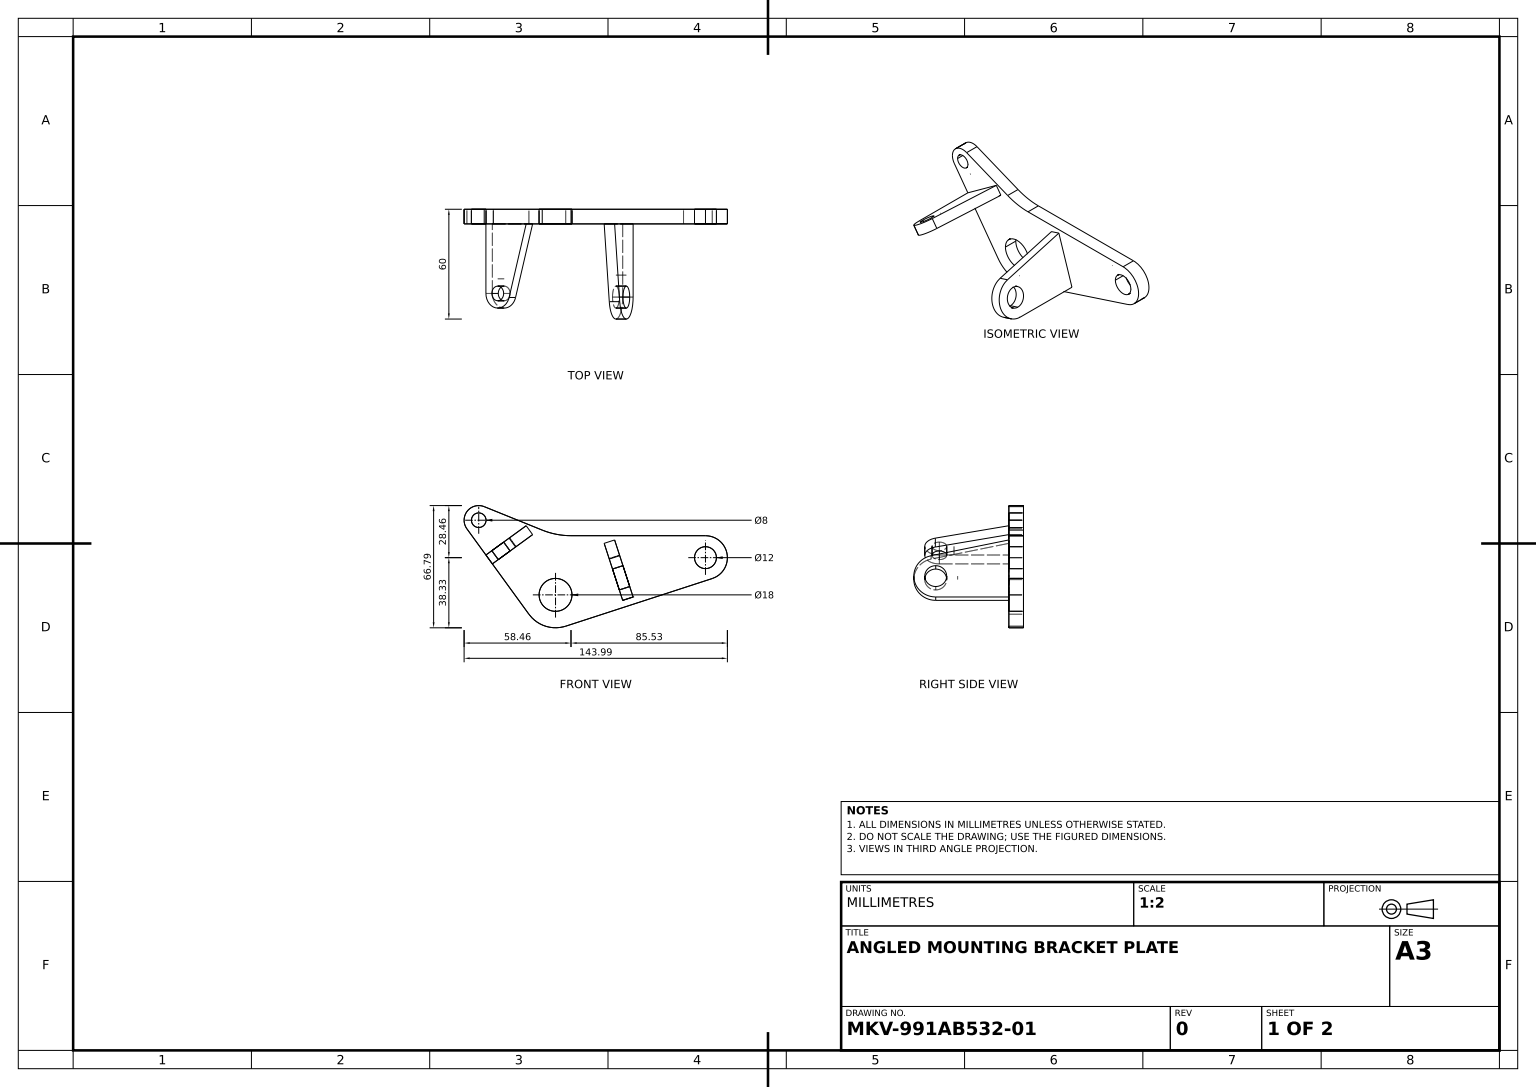
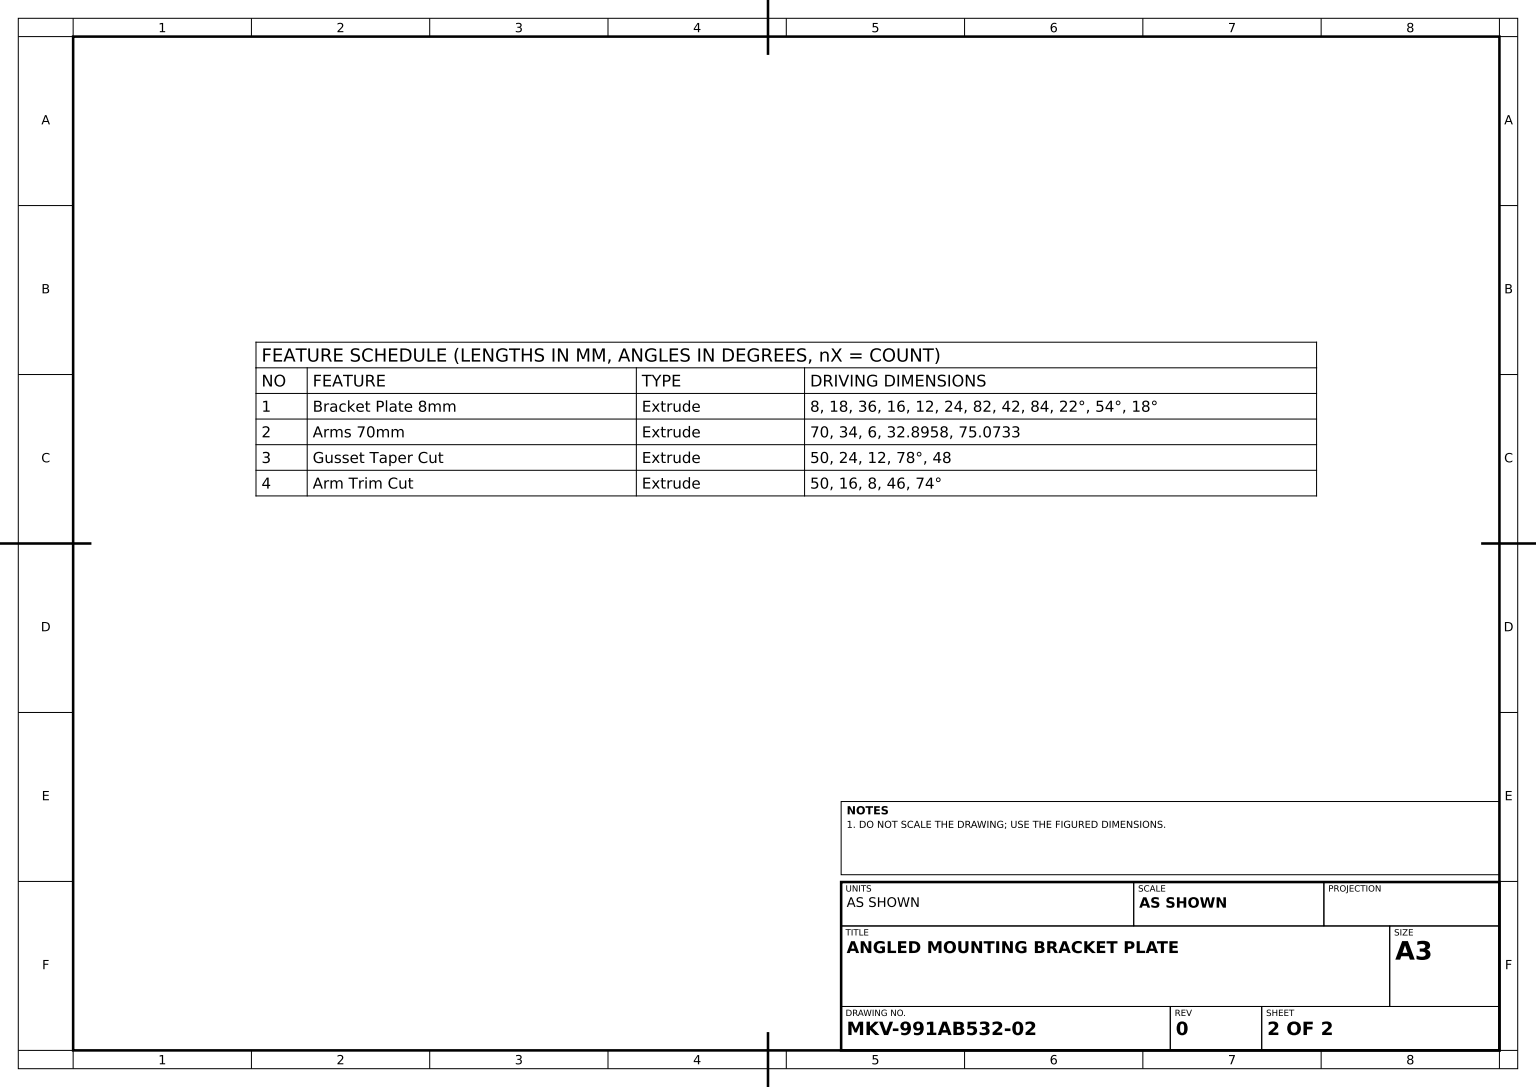
SolidWorks part; units mm, degrees
material "Plain Carbon Steel"
ref_plane "Front Plane" through (0, 0, 0) normal (0, 0, 1) x (1, 0, 0)
ref_plane "Top Plane" through (0, 0, 0) normal (0, 1, 0) x (1, 0, 0)
ref_plane "Right Plane" through (0, 0, 0) normal (1, 0, 0) x (0, 0, -1)
sketch "Bracket Plate Profile" plane through (0, 0, 0) normal (0, 0, 1) x (1, 0, 0)
  line L0 (-48.4721, 36.0927) -> (-14.5623, -10.5801)
  line L1 (5.5623, -17.119) -> (85.7082, 8.922)
  line L3 (-39.0031, 48.2125) -> (-7.2736, 35.3929)
  line L4 (8.4599, 32.3346) -> (82, 32.3346)
  circle A0 centre (0, 0) radius 9
  arc A1 (-14.5623, -10.5801) -> (5.5623, -17.119) centre (0, 0) ccw
  arc A2 (-39.0031, 48.2125) -> (-48.4721, 36.0927) centre (-42, 40.795) ccw
  circle A3 centre (-42, 40.795) radius 4
  arc A4 (85.7082, 8.922) -> (82, 32.3346) centre (82, 20.3346) ccw
  circle A5 centre (82, 20.3346) radius 6
  arc A6 (-7.2736, 35.3929) -> (8.4599, 32.3346) centre (8.4599, 74.3346) ccw
  dimension "D1" = 18
  dimension "D2" = 36
  dimension "D3" = 8
  dimension "D4" = 16
  dimension "D5" = 12
  dimension "D6" = 24
  dimension "D9" = 84
  dimension "D7" = 82
  dimension "D8" = 42
  dimension "D10" = 42
  dimension "D11" = 22
  dimension "D12" = 54
  dimension "D13" = 18
extrude "Bracket Plate 8mm" add sketch "Bracket Plate Profile" along normal blind 8
sketch "Arm Sections 34x6" plane through (0, 0, 8) normal (0, 0, 1) x (1, 0, 0)
  line L0 (37.8982, -6.6124) -> (43.6046, -4.7583)
  line L1 (37.8982, -6.6124) -> (26.6012, 28.1564)
  line L2 (43.6046, -4.7583) -> (32.3075, 30.0105)
  line L3 (26.6012, 28.1564) -> (32.3075, 30.0105)
  line L4 (-38.0737, 21.7805) -> (-34.547, 16.9264)
  line L5 (-38.0737, 21.7805) -> (-15.5763, 38.1259)
  line L6 (-34.547, 16.9264) -> (-12.0496, 33.2718)
  line L7 (-15.5763, 38.1259) -> (-12.0496, 33.2718)
  line L10 (-48.4721, 36.0927) -> (-14.5623, -10.5801) construction
  line L11 (5.5623, -17.119) -> (85.7082, 8.922) construction
  dimension "D1" = 34
  dimension "D2" = 6
  dimension "D3" = 34
  dimension "D4" = 6
  dimension "D5" = 32.8958
  dimension "D6" = 75.0733
extrude "Arms 70mm" add sketch "Arm Sections 34x6" along normal blind 70
sketch "Gusset Taper Cut Profile" plane through (38.0423, 12.3607, 0) normal (0.9511, 0.309, 0) x (0, 0, -1)
  line L0 (-8, 18.5581) -> (-50.4949, 9.5255)
  line L1 (-8, -14.2123) -> (-48, -14.2123)
  line L3 (-8, -18) -> (-8, 18.5581) construction
  line L8 (0, -18) -> (0, 5.4127) construction
  line L10 (-8, -18) -> (-8, 18.5581)
  line L11 (-8, 18.5581) -> (-78, 18.5581)
  line L12 (-78, 18.5581) -> (-78, -18)
  line L13 (-78, -18) -> (-8, -18)
  line L14 (-8, -18) -> (-8, 18.5581)
  line L15 (-8, 18.5581) -> (-78, 18.5581)
  line L16 (-78, 18.5581) -> (-78, -18)
  line L17 (-78, -18) -> (-8, -18)
  circle A0 centre (-48, -2.2123) radius 6
  arc A1 (-50.4949, 9.5255) -> (-48, -14.2123) centre (-48, -2.2123) ccw
  line M4 (-8, -18) -> (-8, 18.5581)
  line M5 (-8, 18.5581) -> (-78, 18.5581)
  line M6 (-78, 18.5581) -> (-78, -18)
  line M7 (-78, -18) -> (-8, -18)
  dimension "D1" = 24
  dimension "D2" = 12
  dimension "D3" = 78
  dimension "D4" = 48
  dimension "D5" = 0
extrude "Gusset Taper Cut" cut sketch "Gusset Taper Cut Profile" against normal blind 50 contours A1 L0 L1 M5 M6 M7 M4 | A0
sketch "Arm Trim Cut Profile" plane through (-23.5114, 32.3607, 0) normal (-0.5878, 0.809, 0) x (0.809, 0.5878, 0)
  line L0 (9.2187, -8) -> (-2.3099, -48.2051)
  line L1 (-18, -8) -> (-18, -46)
  line L4 (-3.2156, 0) -> (-18, 0) construction
  line L8 (9.8083, -8) -> (-18, -8)
  line L9 (-18, -8) -> (-18, -78)
  line L10 (-18, -78) -> (9.8083, -78)
  line L11 (9.8083, -78) -> (9.8083, -8)
  line L12 (9.8083, -8) -> (-18, -8)
  line L13 (-18, -8) -> (-18, -78)
  line L14 (-18, -78) -> (9.8083, -78)
  line L15 (9.8083, -78) -> (9.8083, -8)
  circle A0 centre (-10, -46) radius 4
  circle A1 centre (-10, -46) radius 8
  line M5 (9.8083, -8) -> (-18, -8)
  line M6 (-18, -8) -> (-18, -78)
  line M7 (-18, -78) -> (9.8083, -78)
  line M8 (9.8083, -78) -> (9.8083, -8)
  dimension "D1" = 16
  dimension "D2" = 8
  dimension "D6" = 0
  dimension "D3" = 74
  dimension "D4" = 8
  dimension "D5" = 46
extrude "Arm Trim Cut" cut sketch "Arm Trim Cut Profile" against normal blind 50 contours A0 | A1 L0 M6 M7 M8 M5
